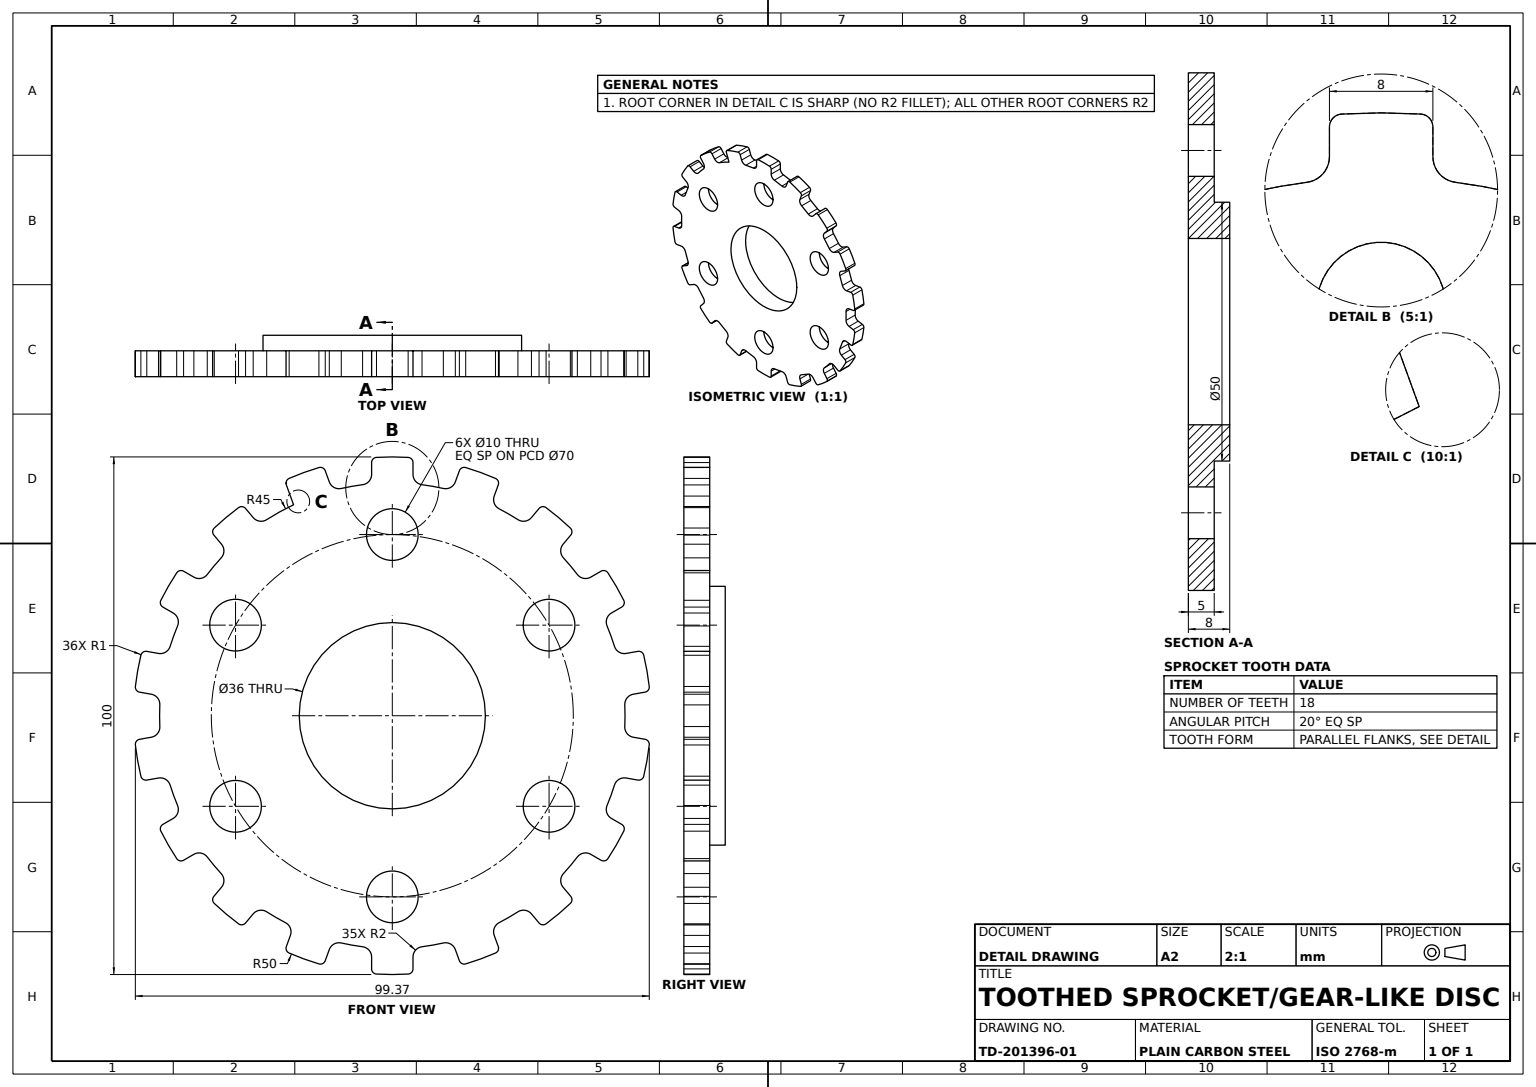
from build123d import *

# Parameters (mm, degrees)
SPROCKET_PLATE_18T_DEPTH = 5
PLATE_HOLES_SKETCH_R     = 5
PLATE_HOLES_CUT_DEPTH    = 71.730230301
BACK_BOSS_SKETCH_R       = 25
BACK_BOSS_3MM_DEPTH      = 3
BACK_BOSS_CUT_SKETCH_R   = 18
BACK_BOSS_CUT_DEPTH      = 72.005390489
PLATE_FILLET_R2_R        = 2
PLATE_FILLET_R1_R        = 1


with BuildPart() as part:
    # Sprocket Profile 18T Sketch → Sprocket Plate 18T (new body)
    with BuildSketch(Plane.XY):
        with BuildLine():
            Line((4, 44.821869662), (4, 49.839743178))
            ThreePointArc((4, 49.839743178), (0, 50), (-4, 49.839743178))
            Line((-4, 49.839743178), (-4, 44.821869662))
            ThreePointArc((-4, 44.821869662), (-7.814167995, 44.316348886), (-11.571211803, 43.486860745))
            Line((-11.571211803, 43.486860745), (-13.287425622, 48.202119459))
            ThreePointArc((-13.287425622, 48.202119459), (-17.101007166, 46.984631039), (-20.804966588, 45.465958312))
            Line((-20.804966588, 45.465958312), (-19.088752769, 40.750699598))
            ThreePointArc((-19.088752769, 40.750699598), (-22.5, 38.97114317), (-25.746764689, 36.906694624))
            Line((-25.746764689, 36.906694624), (-28.972191612, 40.750608746))
            ThreePointArc((-28.972191612, 40.750608746), (-32.139380484, 38.302222156), (-35.100547157, 35.608307869))
            Line((-35.100547157, 35.608307869), (-31.875120234, 31.764393746))
            ThreePointArc((-31.875120234, 31.764393746), (-34.47199994, 28.925442436), (-36.816877772, 25.875036446))
            Line((-36.816877772, 25.875036446), (-41.16248371, 28.383973204))
            ThreePointArc((-41.16248371, 28.383973204), (-43.301270189, 25), (-45.16248371, 21.455769974))
            Line((-45.16248371, 21.455769974), (-40.816877772, 18.946833216))
            ThreePointArc((-40.816877772, 18.946833216), (-42.286167935, 15.39090645), (-43.446332037, 11.722466998))
            Line((-43.446332037, 11.722466998), (-48.387972779, 12.59381159))
            ThreePointArc((-48.387972779, 12.59381159), (-49.240387651, 8.682408883), (-49.7771582, 4.715349566))
            Line((-49.7771582, 4.715349566), (-44.835517458, 3.844004974))
            ThreePointArc((-44.835517458, 3.844004974), (-45, 0), (-44.835517458, -3.844004974))
            Line((-44.835517458, -3.844004974), (-49.7771582, -4.715349566))
            ThreePointArc((-49.7771582, -4.715349566), (-49.240387651, -8.682408883), (-48.387972779, -12.59381159))
            Line((-48.387972779, -12.59381159), (-43.446332037, -11.722466998))
            ThreePointArc((-43.446332037, -11.722466998), (-42.286167935, -15.39090645), (-40.816877772, -18.946833216))
            Line((-40.816877772, -18.946833216), (-45.16248371, -21.455769974))
            ThreePointArc((-45.16248371, -21.455769974), (-43.301270189, -25), (-41.16248371, -28.383973204))
            Line((-41.16248371, -28.383973204), (-36.816877772, -25.875036446))
            ThreePointArc((-36.816877772, -25.875036446), (-34.47199994, -28.925442436), (-31.875120234, -31.764393746))
            Line((-31.875120234, -31.764393746), (-35.100547157, -35.608307869))
            ThreePointArc((-35.100547157, -35.608307869), (-32.139380484, -38.302222156), (-28.972191612, -40.750608746))
            Line((-28.972191612, -40.750608746), (-25.746764689, -36.906694624))
            ThreePointArc((-25.746764689, -36.906694624), (-22.5, -38.97114317), (-19.088752769, -40.750699598))
            Line((-19.088752769, -40.750699598), (-20.804966588, -45.465958312))
            ThreePointArc((-20.804966588, -45.465958312), (-17.101007166, -46.984631039), (-13.287425622, -48.202119459))
            Line((-13.287425622, -48.202119459), (-11.571211803, -43.486860745))
            ThreePointArc((-11.571211803, -43.486860745), (-7.814167995, -44.316348886), (-4, -44.821869662))
            Line((-4, -44.821869662), (-4, -49.839743178))
            ThreePointArc((-4, -49.839743178), (0, -50), (4, -49.839743178))
            Line((4, -49.839743178), (4, -44.821869662))
            ThreePointArc((4, -44.821869662), (7.814167995, -44.316348886), (11.571211803, -43.486860745))
            Line((11.571211803, -43.486860745), (13.287425622, -48.202119459))
            ThreePointArc((13.287425622, -48.202119459), (17.101007166, -46.984631039), (20.804966588, -45.465958312))
            Line((20.804966588, -45.465958312), (19.088752769, -40.750699598))
            ThreePointArc((19.088752769, -40.750699598), (22.5, -38.97114317), (25.746764689, -36.906694624))
            Line((25.746764689, -36.906694624), (28.972191612, -40.750608746))
            ThreePointArc((28.972191612, -40.750608746), (32.139380484, -38.302222156), (35.100547157, -35.608307869))
            Line((35.100547157, -35.608307869), (31.875120234, -31.764393746))
            ThreePointArc((31.875120234, -31.764393746), (34.47199994, -28.925442436), (36.816877772, -25.875036446))
            Line((36.816877772, -25.875036446), (41.16248371, -28.383973204))
            ThreePointArc((41.16248371, -28.383973204), (43.301270189, -25), (45.16248371, -21.455769974))
            Line((45.16248371, -21.455769974), (40.816877772, -18.946833216))
            ThreePointArc((40.816877772, -18.946833216), (42.286167935, -15.39090645), (43.446332037, -11.722466998))
            Line((43.446332037, -11.722466998), (48.387972779, -12.59381159))
            ThreePointArc((48.387972779, -12.59381159), (49.240387651, -8.682408883), (49.7771582, -4.715349566))
            Line((49.7771582, -4.715349566), (44.835517458, -3.844004974))
            ThreePointArc((44.835517458, -3.844004974), (45, 0), (44.835517458, 3.844004974))
            Line((44.835517458, 3.844004974), (49.7771582, 4.715349566))
            ThreePointArc((49.7771582, 4.715349566), (49.240387651, 8.682408883), (48.387972779, 12.59381159))
            Line((48.387972779, 12.59381159), (43.446332037, 11.722466998))
            ThreePointArc((43.446332037, 11.722466998), (42.286167935, 15.39090645), (40.816877772, 18.946833216))
            Line((40.816877772, 18.946833216), (45.16248371, 21.455769974))
            ThreePointArc((45.16248371, 21.455769974), (43.301270189, 25), (41.16248371, 28.383973204))
            Line((41.16248371, 28.383973204), (36.816877772, 25.875036446))
            ThreePointArc((36.816877772, 25.875036446), (34.47199994, 28.925442436), (31.875120234, 31.764393746))
            Line((31.875120234, 31.764393746), (35.100547157, 35.608307869))
            ThreePointArc((35.100547157, 35.608307869), (32.139380484, 38.302222156), (28.972191612, 40.750608746))
            Line((28.972191612, 40.750608746), (25.746764689, 36.906694624))
            ThreePointArc((25.746764689, 36.906694624), (22.5, 38.97114317), (19.088752769, 40.750699598))
            Line((19.088752769, 40.750699598), (20.804966588, 45.465958312))
            ThreePointArc((20.804966588, 45.465958312), (17.101007166, 46.984631039), (13.287425622, 48.202119459))
            Line((13.287425622, 48.202119459), (11.571211803, 43.486860745))
            ThreePointArc((11.571211803, 43.486860745), (7.814167995, 44.316348886), (4, 44.821869662))
        make_face()
    extrude(amount=SPROCKET_PLATE_18T_DEPTH)

    # Plate Holes Sketch → Plate Holes Cut (cut, through all)
    with BuildSketch(Plane.XY):
        with Locations((0, 35)):
            Circle(PLATE_HOLES_SKETCH_R)
        with Locations((30.310889132, 17.5)):
            Circle(PLATE_HOLES_SKETCH_R)
        with Locations((30.310889132, -17.5)):
            Circle(PLATE_HOLES_SKETCH_R)
        with Locations((0, -35)):
            Circle(PLATE_HOLES_SKETCH_R)
        with Locations((-30.310889132, -17.5)):
            Circle(PLATE_HOLES_SKETCH_R)
        with Locations((-30.310889132, 17.5)):
            Circle(PLATE_HOLES_SKETCH_R)
    extrude(amount=PLATE_HOLES_CUT_DEPTH, mode=Mode.SUBTRACT)

    # Back Boss Sketch → Back Boss 3mm (add)
    with BuildSketch(Plane(origin=(0, 0, 0), x_dir=(-1, 0, 0), z_dir=(0, 0, -1))):
        with Locations(Location((0, 0, 0), (0, 0, 180))):
            Circle(BACK_BOSS_SKETCH_R)
    extrude(amount=BACK_BOSS_3MM_DEPTH)

    # Back Boss Cut Sketch → Back Boss Cut (cut, through all)
    with BuildSketch(Plane(origin=(0, 0, -3), x_dir=(-1, 0, 0), z_dir=(0, 0, -1))):
        Circle(BACK_BOSS_CUT_SKETCH_R)
    extrude(amount=-BACK_BOSS_CUT_DEPTH, mode=Mode.SUBTRACT)

    # Plate Fillet R2
    plate_fillet_r2_edges = [part.edges().sort_by_distance(p)[0] for p in [
        (11.571211803, 43.486860745, 2.5),
        (19.088752769, 40.750699598, 2.5),
        (25.746764689, 36.906694624, 2.5),
        (31.875120234, 31.764393746, 2.5),
        (36.816877772, 25.875036446, 2.5),
        (40.816877772, 18.946833216, 2.5),
        (43.446332037, 11.722466998, 2.5),
        (44.835517458, 3.844004974, 2.5),
        (44.835517458, -3.844004974, 2.5),
        (43.446332037, -11.722466998, 2.5),
        (40.816877772, -18.946833216, 2.5),
        (36.816877772, -25.875036446, 2.5),
        (31.875120234, -31.764393746, 2.5),
        (25.746764689, -36.906694624, 2.5),
        (19.088752769, -40.750699598, 2.5),
        (11.571211803, -43.486860745, 2.5),
        (4, -44.821869662, 2.5),
        (-4, -44.821869662, 2.5),
        (-11.571211803, -43.486860745, 2.5),
        (-19.088752769, -40.750699598, 2.5),
        (-25.746764689, -36.906694624, 2.5),
        (-31.875120234, -31.764393746, 2.5),
        (-36.816877772, -25.875036446, 2.5),
        (-40.816877772, -18.946833216, 2.5),
        (-43.446332037, -11.722466998, 2.5),
        (-44.835517458, -3.844004974, 2.5),
        (-44.835517458, 3.844004974, 2.5),
        (-43.446332037, 11.722466998, 2.5),
        (-40.816877772, 18.946833216, 2.5),
        (-36.816877772, 25.875036446, 2.5),
        (-31.875120234, 31.764393746, 2.5),
        (-25.746764689, 36.906694624, 2.5),
        (-11.571211803, 43.486860745, 2.5),
        (-4, 44.821869662, 2.5),
        (4, 44.821869662, 2.5),
    ]]
    fillet(plate_fillet_r2_edges, radius=PLATE_FILLET_R2_R)

    # Plate Fillet R1
    plate_fillet_r1_edges = [part.edges().sort_by_distance(p)[0] for p in [
        (13.287425622, 48.202119459, 2.5),
        (20.804966588, 45.465958312, 2.5),
        (28.972191612, 40.750608746, 2.5),
        (35.100547157, 35.608307869, 2.5),
        (41.16248371, 28.383973204, 2.5),
        (45.16248371, 21.455769974, 2.5),
        (48.387972779, 12.59381159, 2.5),
        (49.7771582, 4.715349566, 2.5),
        (49.7771582, -4.715349566, 2.5),
        (48.387972779, -12.59381159, 2.5),
        (45.16248371, -21.455769974, 2.5),
        (41.16248371, -28.383973204, 2.5),
        (35.100547157, -35.608307869, 2.5),
        (28.972191612, -40.750608746, 2.5),
        (20.804966588, -45.465958312, 2.5),
        (13.287425622, -48.202119459, 2.5),
        (4, -49.839743178, 2.5),
        (-4, -49.839743178, 2.5),
        (-13.287425622, -48.202119459, 2.5),
        (-20.804966588, -45.465958312, 2.5),
        (-28.972191612, -40.750608746, 2.5),
        (-35.100547157, -35.608307869, 2.5),
        (-41.16248371, -28.383973204, 2.5),
        (-45.16248371, -21.455769974, 2.5),
        (-48.387972779, -12.59381159, 2.5),
        (-49.7771582, -4.715349566, 2.5),
        (-49.7771582, 4.715349566, 2.5),
        (-48.387972779, 12.59381159, 2.5),
        (-45.16248371, 21.455769974, 2.5),
        (-41.16248371, 28.383973204, 2.5),
        (-35.100547157, 35.608307869, 2.5),
        (-28.972191612, 40.750608746, 2.5),
        (-20.804966588, 45.465958312, 2.5),
        (-13.287425622, 48.202119459, 2.5),
        (-4, 49.839743178, 2.5),
        (4, 49.839743178, 2.5),
    ]]
    fillet(plate_fillet_r1_edges, radius=PLATE_FILLET_R1_R)


solid = part.part
